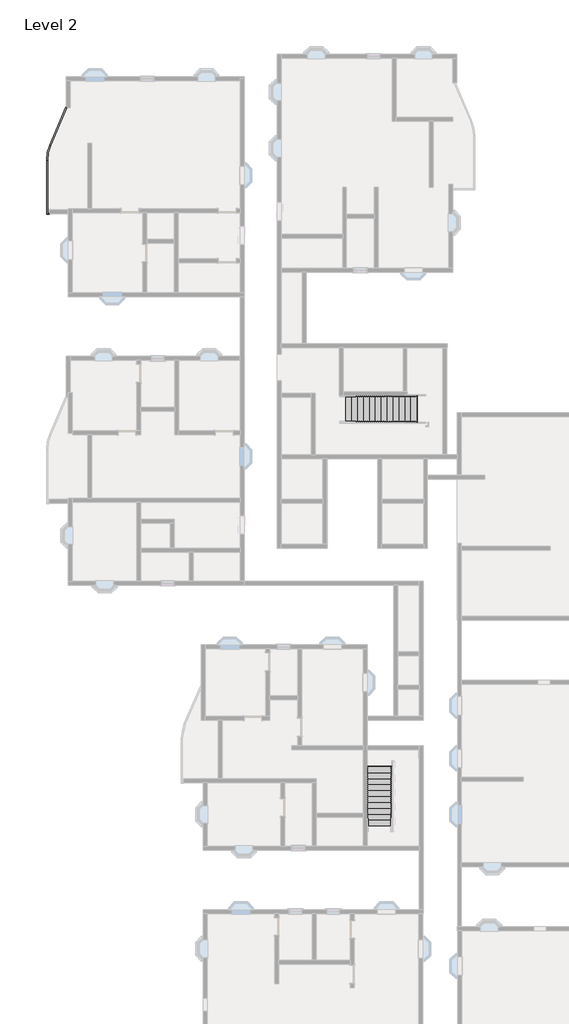
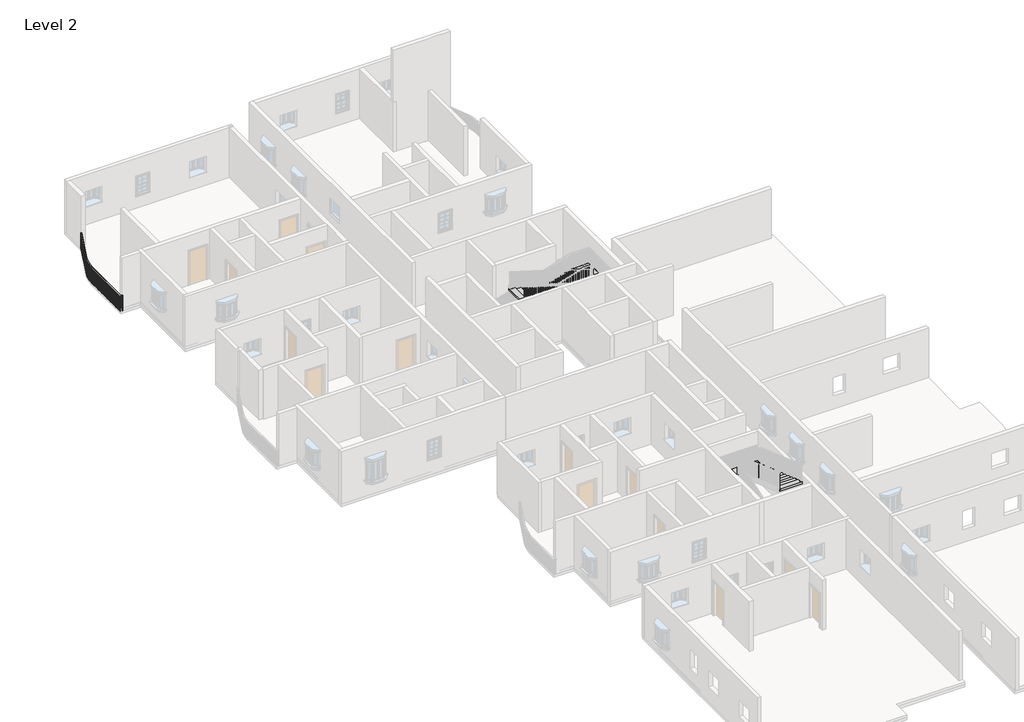
# One storey, part 12 of 14: 2 stair flights, 1 railing.
"""IFC4 building model written with IfcOpenShell, lengths in millimetres."""

from ifc_helpers import new_model, si_unit, frame, origin, place, context, project, spatial, polyline, circle_curve, outline, extrude, transform, mapped, element, save
from ifc_brep_helpers import plane_surface, cylinder_surface, revolved_surface, advanced_brep
from components import stair_flight_f6874503, stair_flight_175a6785

model = new_model("IFC4")

# Units and contexts
model_context = context("Model", 3, world=origin())
ifc_project = project(units=[si_unit("LENGTHUNIT", "METRE", prefix="MILLI")], contexts=[model_context])

# Site, building, storey
site = spatial("IfcSite", under=ifc_project)
building = spatial("IfcBuilding", under=site)
storey = spatial("IfcBuildingStorey", under=building, Name="Level 2", Elevation=3048.0)

# Railing
placement = place(None, origin())
element("IfcRailing", 1, ObjectType="Handrail - Rectangular", at=placement, inside=storey, context=model_context, shape_type="SolidModel", body=[
    advanced_brep(
    [(-19327.739878, 27355.8257339, 3962.4), (-19327.739878, 27355.8257339, 3911.6), (-19374.4383922, 27375.822953, 3911.6), (-19374.4383922, 27375.822953, 3962.4), (-20162.483418, 25406.4905323, 3962.4), (-20162.483418, 25406.4905323, 3911.6), (-20209.1819322, 25426.4877514, 3911.6), (-20209.1819322, 25426.4877514, 3962.4), (-20316.2891351, 24656.5948172, 3911.6), (-20316.2891351, 24656.5948172, 3962.4), (-20367.0891351, 24656.5948172, 3911.6), (-20367.0891351, 24656.5948172, 3962.4), (-20316.2891351, 21915.0583494, 3962.4), (-20316.2891351, 21915.0583494, 3911.6), (-20367.0891351, 21864.2583494, 3911.6), (-20367.0891351, 21864.2583494, 3962.4), (-20240.0891351, 21915.0583494, 3962.4), (-20240.0891351, 21864.2583494, 3962.4), (-20240.0891351, 21864.2583494, 3911.6), (-20240.0891351, 21915.0583494, 3911.6)],
    [
        (0, 1),
        (1, 2),
        (2, 3),
        (3, 0),
        (0, 4),
        (4, 5),
        (5, 1),
        (5, 6),
        (6, 2),
        (6, 7),
        (7, 3),
        (7, 4),
        (8, 5, circle_curve(frame((-18411.2891351, 24656.5948172, 3911.6), z_axis=(0.0, 0.0, -1.0), x_axis=(-0.9192620907623796, 0.39364604467361086, 0.0)), 1905.0)),
        (4, 9, circle_curve(frame((-18411.2891351, 24656.5948172, 3962.4), z_axis=(0.0, 0.0, 1.0), x_axis=(-0.9192620907623796, 0.39364604467361086, 0.0)), 1905.0)),
        (9, 8),
        (10, 6, circle_curve(frame((-18411.2891351, 24656.5948172, 3911.6), z_axis=(0.0, 0.0, -1.0), x_axis=(-0.9192620907623796, 0.39364604467361086, 0.0)), 1955.8)),
        (8, 10),
        (11, 7, circle_curve(frame((-18411.2891351, 24656.5948172, 3962.4), z_axis=(0.0, 0.0, -1.0), x_axis=(-0.9192620907623796, 0.39364604467361086, 0.0)), 1955.8)),
        (10, 11),
        (11, 9),
        (9, 12),
        (12, 13),
        (13, 8),
        (13, 14),
        (14, 10),
        (14, 15),
        (15, 11),
        (15, 12),
        (16, 17),
        (17, 18),
        (18, 19),
        (19, 16),
        (12, 16),
        (19, 13),
        (18, 14),
        (17, 15),
    ],
    [
        plane_surface(frame((-19351.0891351, 27365.8243434, 3962.4), z_axis=(0.3936460446736102, 0.91926209076238, 0.0), x_axis=(0.91926209076238, -0.3936460446736102, 0.0))),
        plane_surface(frame((-19327.739878, 27355.8257339, 3962.4), z_axis=(0.9192620907623803, -0.39364604467360953, 0.0), x_axis=(-0.39364604467360953, -0.9192620907623803, 0.0))),
        plane_surface(frame((-19327.739878, 27355.8257339, 3911.6), z_axis=(0.0, 0.0, -1.0), x_axis=(-0.39364604467360953, -0.9192620907623803, 0.0))),
        plane_surface(frame((-19374.4383922, 27375.822953, 3911.6), z_axis=(-0.9192620907623803, 0.39364604467360953, 0.0), x_axis=(-0.39364604467360953, -0.9192620907623803, 0.0))),
        plane_surface(frame((-19374.4383922, 27375.822953, 3962.4), z_axis=(0.0, 0.0, 1.0), x_axis=(-0.39364604467360953, -0.9192620907623803, 0.0))),
        revolved_surface(polyline([(-20162.48341800233, 25406.49053230323, 3962.4), (-20162.48341800233, 25406.49053230323, 3911.6)]), (-18411.2891351, 24656.5948172, 3962.4), (0.0, 0.0, 1.0)),
        plane_surface(frame((-18411.2891351, 24656.5948172, 3911.6), z_axis=(0.0, 0.0, -1.0000000000000002), x_axis=(-0.9192620907623797, 0.3936460446736109, 0.0))),
        cylinder_surface(frame((-18411.2891351, 24656.5948172, 3962.4), z_axis=(0.0, 0.0, 1.0), x_axis=(-0.9192620907623796, 0.39364604467361086, 0.0)), 1955.8),
        plane_surface(frame((-18411.2891351, 24656.5948172, 3962.4), z_axis=(0.0, 0.0, 1.0000000000000002), x_axis=(-0.9192620907623797, 0.3936460446736109, 0.0))),
        plane_surface(frame((-20316.2891351, 24656.5948172, 3962.4), z_axis=(1.0, 0.0, 0.0), x_axis=(0.0, -1.0, 0.0))),
        plane_surface(frame((-20316.2891351, 24656.5948172, 3911.6), z_axis=(0.0, 0.0, -1.0), x_axis=(0.0, -1.0, 0.0))),
        plane_surface(frame((-20367.0891351, 24656.5948172, 3911.6), z_axis=(-1.0, 0.0, 0.0), x_axis=(0.0, -1.0, 0.0))),
        plane_surface(frame((-20367.0891351, 24656.5948172, 3962.4), z_axis=(0.0, 0.0, 1.0), x_axis=(0.0, -1.0, 0.0))),
        plane_surface(frame((-20240.0891351, 21889.6583494, 3962.4), z_axis=(1.0, 0.0, 0.0), x_axis=(0.0, 1.0, 0.0))),
        plane_surface(frame((-20316.2891351, 21915.0583494, 3962.4), z_axis=(0.0, 1.0, 0.0), x_axis=(1.0, 0.0, 0.0))),
        plane_surface(frame((-20316.2891351, 21915.0583494, 3911.6), z_axis=(0.0, 0.0, -1.0), x_axis=(1.0, 0.0, 0.0))),
        plane_surface(frame((-20367.0891351, 21864.2583494, 3911.6), z_axis=(0.0, -1.0, 0.0), x_axis=(1.0, 0.0, 0.0))),
        plane_surface(frame((-20367.0891351, 21864.2583494, 3962.4), z_axis=(0.0, 0.0, 1.0), x_axis=(1.0, 0.0, 0.0))),
    ],
    [
        (0, [[1, 2, 3, 4]]),
        (1, [[-1, 5, 6, 7]]),
        (2, [[-2, -7, 8, 9]]),
        (3, [[-3, -9, 10, 11]]),
        (4, [[-4, -11, 12, -5]]),
        (5, [[13, -6, 14, 15]]),
        (6, [[16, -8, -13, 17]]),
        (7, [[18, -10, -16, 19]]),
        (8, [[-14, -12, -18, 20]]),
        (9, [[-15, 21, 22, 23]]),
        (10, [[-17, -23, 24, 25]]),
        (11, [[-19, -25, 26, 27]]),
        (12, [[-20, -27, 28, -21]]),
        (13, [[29, 30, 31, 32]]),
        (14, [[-22, 33, -32, 34]]),
        (15, [[-24, -34, -31, 35]]),
        (16, [[-26, -35, -30, 36]]),
        (17, [[-28, -36, -29, -33]]),
    ],
),
    extrude(outline(polyline([(-20351.2141351, 21922.9198172), (-20332.1641351, 21922.9198172), (-20332.1641351, 21903.8698172), (-20351.2141351, 21903.8698172), (-20351.2141351, 21922.9198172)])), frame((0.0, 0.0, 3048.0), z_axis=(0.0, 0.0, 1.0), x_axis=(1.0, 0.0, 0.0)), (0.0, 0.0, 1.0), 863.6),
    extrude(outline(polyline([(-20351.2141351, 22024.5198172), (-20332.1641351, 22024.5198172), (-20332.1641351, 22005.4698172), (-20351.2141351, 22005.4698172), (-20351.2141351, 22024.5198172)])), frame((0.0, 0.0, 3048.0), z_axis=(0.0, 0.0, 1.0), x_axis=(1.0, 0.0, 0.0)), (0.0, 0.0, 1.0), 863.6),
    extrude(outline(polyline([(-20351.2141351, 22126.1198172), (-20332.1641351, 22126.1198172), (-20332.1641351, 22107.0698172), (-20351.2141351, 22107.0698172), (-20351.2141351, 22126.1198172)])), frame((0.0, 0.0, 3048.0), z_axis=(0.0, 0.0, 1.0), x_axis=(1.0, 0.0, 0.0)), (0.0, 0.0, 1.0), 863.6),
    extrude(outline(polyline([(-20351.2141351, 22227.7198172), (-20332.1641351, 22227.7198172), (-20332.1641351, 22208.6698172), (-20351.2141351, 22208.6698172), (-20351.2141351, 22227.7198172)])), frame((0.0, 0.0, 3048.0), z_axis=(0.0, 0.0, 1.0), x_axis=(1.0, 0.0, 0.0)), (0.0, 0.0, 1.0), 863.6),
    extrude(outline(polyline([(-20351.2141351, 22329.3198172), (-20332.1641351, 22329.3198172), (-20332.1641351, 22310.2698172), (-20351.2141351, 22310.2698172), (-20351.2141351, 22329.3198172)])), frame((0.0, 0.0, 3048.0), z_axis=(0.0, 0.0, 1.0), x_axis=(1.0, 0.0, 0.0)), (0.0, 0.0, 1.0), 863.6),
    extrude(outline(polyline([(-20351.2141351, 22430.9198172), (-20332.1641351, 22430.9198172), (-20332.1641351, 22411.8698172), (-20351.2141351, 22411.8698172), (-20351.2141351, 22430.9198172)])), frame((0.0, 0.0, 3048.0), z_axis=(0.0, 0.0, 1.0), x_axis=(1.0, 0.0, 0.0)), (0.0, 0.0, 1.0), 863.6),
    extrude(outline(polyline([(-20351.2141351, 22532.5198172), (-20332.1641351, 22532.5198172), (-20332.1641351, 22513.4698172), (-20351.2141351, 22513.4698172), (-20351.2141351, 22532.5198172)])), frame((0.0, 0.0, 3048.0), z_axis=(0.0, 0.0, 1.0), x_axis=(1.0, 0.0, 0.0)), (0.0, 0.0, 1.0), 863.6),
    extrude(outline(polyline([(-20351.2141351, 22634.1198172), (-20332.1641351, 22634.1198172), (-20332.1641351, 22615.0698172), (-20351.2141351, 22615.0698172), (-20351.2141351, 22634.1198172)])), frame((0.0, 0.0, 3048.0), z_axis=(0.0, 0.0, 1.0), x_axis=(1.0, 0.0, 0.0)), (0.0, 0.0, 1.0), 863.6),
    extrude(outline(polyline([(-20351.2141351, 22735.7198172), (-20332.1641351, 22735.7198172), (-20332.1641351, 22716.6698172), (-20351.2141351, 22716.6698172), (-20351.2141351, 22735.7198172)])), frame((0.0, 0.0, 3048.0), z_axis=(0.0, 0.0, 1.0), x_axis=(1.0, 0.0, 0.0)), (0.0, 0.0, 1.0), 863.6),
    extrude(outline(polyline([(-20351.2141351, 22837.3198172), (-20332.1641351, 22837.3198172), (-20332.1641351, 22818.2698172), (-20351.2141351, 22818.2698172), (-20351.2141351, 22837.3198172)])), frame((0.0, 0.0, 3048.0), z_axis=(0.0, 0.0, 1.0), x_axis=(1.0, 0.0, 0.0)), (0.0, 0.0, 1.0), 863.6),
    extrude(outline(polyline([(-20351.2141351, 22938.9198172), (-20332.1641351, 22938.9198172), (-20332.1641351, 22919.8698172), (-20351.2141351, 22919.8698172), (-20351.2141351, 22938.9198172)])), frame((0.0, 0.0, 3048.0), z_axis=(0.0, 0.0, 1.0), x_axis=(1.0, 0.0, 0.0)), (0.0, 0.0, 1.0), 863.6),
    extrude(outline(polyline([(-20351.2141351, 23040.5198172), (-20332.1641351, 23040.5198172), (-20332.1641351, 23021.4698172), (-20351.2141351, 23021.4698172), (-20351.2141351, 23040.5198172)])), frame((0.0, 0.0, 3048.0), z_axis=(0.0, 0.0, 1.0), x_axis=(1.0, 0.0, 0.0)), (0.0, 0.0, 1.0), 863.6),
    extrude(outline(polyline([(-20351.2141351, 23142.1198172), (-20332.1641351, 23142.1198172), (-20332.1641351, 23123.0698172), (-20351.2141351, 23123.0698172), (-20351.2141351, 23142.1198172)])), frame((0.0, 0.0, 3048.0), z_axis=(0.0, 0.0, 1.0), x_axis=(1.0, 0.0, 0.0)), (0.0, 0.0, 1.0), 863.6),
    extrude(outline(polyline([(-20351.2141351, 23243.7198172), (-20332.1641351, 23243.7198172), (-20332.1641351, 23224.6698172), (-20351.2141351, 23224.6698172), (-20351.2141351, 23243.7198172)])), frame((0.0, 0.0, 3048.0), z_axis=(0.0, 0.0, 1.0), x_axis=(1.0, 0.0, 0.0)), (0.0, 0.0, 1.0), 863.6),
    extrude(outline(polyline([(-20351.2141351, 23345.3198172), (-20332.1641351, 23345.3198172), (-20332.1641351, 23326.2698172), (-20351.2141351, 23326.2698172), (-20351.2141351, 23345.3198172)])), frame((0.0, 0.0, 3048.0), z_axis=(0.0, 0.0, 1.0), x_axis=(1.0, 0.0, 0.0)), (0.0, 0.0, 1.0), 863.6),
    extrude(outline(polyline([(-20351.2141351, 23446.9198172), (-20332.1641351, 23446.9198172), (-20332.1641351, 23427.8698172), (-20351.2141351, 23427.8698172), (-20351.2141351, 23446.9198172)])), frame((0.0, 0.0, 3048.0), z_axis=(0.0, 0.0, 1.0), x_axis=(1.0, 0.0, 0.0)), (0.0, 0.0, 1.0), 863.6),
    extrude(outline(polyline([(-20351.2141351, 23548.5198172), (-20332.1641351, 23548.5198172), (-20332.1641351, 23529.4698172), (-20351.2141351, 23529.4698172), (-20351.2141351, 23548.5198172)])), frame((0.0, 0.0, 3048.0), z_axis=(0.0, 0.0, 1.0), x_axis=(1.0, 0.0, 0.0)), (0.0, 0.0, 1.0), 863.6),
    extrude(outline(polyline([(-20351.2141351, 23650.1198172), (-20332.1641351, 23650.1198172), (-20332.1641351, 23631.0698172), (-20351.2141351, 23631.0698172), (-20351.2141351, 23650.1198172)])), frame((0.0, 0.0, 3048.0), z_axis=(0.0, 0.0, 1.0), x_axis=(1.0, 0.0, 0.0)), (0.0, 0.0, 1.0), 863.6),
    extrude(outline(polyline([(-20351.2141351, 23751.7198172), (-20332.1641351, 23751.7198172), (-20332.1641351, 23732.6698172), (-20351.2141351, 23732.6698172), (-20351.2141351, 23751.7198172)])), frame((0.0, 0.0, 3048.0), z_axis=(0.0, 0.0, 1.0), x_axis=(1.0, 0.0, 0.0)), (0.0, 0.0, 1.0), 863.6),
    extrude(outline(polyline([(-20351.2141351, 23853.3198172), (-20332.1641351, 23853.3198172), (-20332.1641351, 23834.2698172), (-20351.2141351, 23834.2698172), (-20351.2141351, 23853.3198172)])), frame((0.0, 0.0, 3048.0), z_axis=(0.0, 0.0, 1.0), x_axis=(1.0, 0.0, 0.0)), (0.0, 0.0, 1.0), 863.6),
    extrude(outline(polyline([(-20351.2141351, 23954.9198172), (-20332.1641351, 23954.9198172), (-20332.1641351, 23935.8698172), (-20351.2141351, 23935.8698172), (-20351.2141351, 23954.9198172)])), frame((0.0, 0.0, 3048.0), z_axis=(0.0, 0.0, 1.0), x_axis=(1.0, 0.0, 0.0)), (0.0, 0.0, 1.0), 863.6),
    extrude(outline(polyline([(-20351.2141351, 24056.5198172), (-20332.1641351, 24056.5198172), (-20332.1641351, 24037.4698172), (-20351.2141351, 24037.4698172), (-20351.2141351, 24056.5198172)])), frame((0.0, 0.0, 3048.0), z_axis=(0.0, 0.0, 1.0), x_axis=(1.0, 0.0, 0.0)), (0.0, 0.0, 1.0), 863.6),
    extrude(outline(polyline([(-20351.2141351, 24158.1198172), (-20332.1641351, 24158.1198172), (-20332.1641351, 24139.0698172), (-20351.2141351, 24139.0698172), (-20351.2141351, 24158.1198172)])), frame((0.0, 0.0, 3048.0), z_axis=(0.0, 0.0, 1.0), x_axis=(1.0, 0.0, 0.0)), (0.0, 0.0, 1.0), 863.6),
    extrude(outline(polyline([(-20351.2141351, 24259.7198172), (-20332.1641351, 24259.7198172), (-20332.1641351, 24240.6698172), (-20351.2141351, 24240.6698172), (-20351.2141351, 24259.7198172)])), frame((0.0, 0.0, 3048.0), z_axis=(0.0, 0.0, 1.0), x_axis=(1.0, 0.0, 0.0)), (0.0, 0.0, 1.0), 863.6),
    extrude(outline(polyline([(-20351.2141351, 24361.3198172), (-20332.1641351, 24361.3198172), (-20332.1641351, 24342.2698172), (-20351.2141351, 24342.2698172), (-20351.2141351, 24361.3198172)])), frame((0.0, 0.0, 3048.0), z_axis=(0.0, 0.0, 1.0), x_axis=(1.0, 0.0, 0.0)), (0.0, 0.0, 1.0), 863.6),
    extrude(outline(polyline([(-20351.2141351, 24462.9198172), (-20332.1641351, 24462.9198172), (-20332.1641351, 24443.8698172), (-20351.2141351, 24443.8698172), (-20351.2141351, 24462.9198172)])), frame((0.0, 0.0, 3048.0), z_axis=(0.0, 0.0, 1.0), x_axis=(1.0, 0.0, 0.0)), (0.0, 0.0, 1.0), 863.6),
    extrude(outline(polyline([(-20351.2141351, 24564.5198172), (-20332.1641351, 24564.5198172), (-20332.1641351, 24545.4698172), (-20351.2141351, 24545.4698172), (-20351.2141351, 24564.5198172)])), frame((0.0, 0.0, 3048.0), z_axis=(0.0, 0.0, 1.0), x_axis=(1.0, 0.0, 0.0)), (0.0, 0.0, 1.0), 863.6),
    extrude(outline(polyline([(-20349.6005818, 24736.2720848), (-20330.5630441, 24735.5831307), (-20331.2519982, 24716.545593), (-20350.289536, 24717.2345471), (-20349.6005818, 24736.2720848)])), frame((0.0, 0.0, 3048.0), z_axis=(0.0, 0.0, 1.0), x_axis=(1.0, 0.0, 0.0)), (0.0, 0.0, 1.0), 863.6),
    extrude(outline(polyline([(-20342.724955, 24838.1310534), (-20323.750023, 24836.4415402), (-20325.4395363, 24817.4666081), (-20344.4144683, 24819.1561214), (-20342.724955, 24838.1310534)])), frame((0.0, 0.0, 3048.0), z_axis=(0.0, 0.0, 1.0), x_axis=(1.0, 0.0, 0.0)), (0.0, 0.0, 1.0), 863.6),
    extrude(outline(polyline([(-20330.5003254, 24939.4872677), (-20311.6405491, 24936.8018743), (-20314.3259425, 24917.942098), (-20333.1857188, 24920.6274914), (-20330.5003254, 24939.4872677)])), frame((0.0, 0.0, 3048.0), z_axis=(0.0, 0.0, 1.0), x_axis=(1.0, 0.0, 0.0)), (0.0, 0.0, 1.0), 863.6),
    extrude(outline(polyline([(-20312.9605484, 25040.0600272), (-20294.2681589, 25036.3861907), (-20297.9419954, 25017.6938012), (-20316.6343849, 25021.3676377), (-20312.9605484, 25040.0600272)])), frame((0.0, 0.0, 3048.0), z_axis=(0.0, 0.0, 1.0), x_axis=(1.0, 0.0, 0.0)), (0.0, 0.0, 1.0), 863.6),
    extrude(outline(polyline([(-20290.1541995, 25139.5708014), (-20271.6809643, 25134.9186963), (-20276.3330693, 25116.4454611), (-20294.8063045, 25121.0975662), (-20290.1541995, 25139.5708014)])), frame((0.0, 0.0, 3048.0), z_axis=(0.0, 0.0, 1.0), x_axis=(1.0, 0.0, 0.0)), (0.0, 0.0, 1.0), 863.6),
    extrude(outline(polyline([(-20262.1444395, 25237.7440008), (-20243.9415192, 25232.1265109), (-20249.5590091, 25213.9235906), (-20267.7619294, 25219.5410805), (-20262.1444395, 25237.7440008)])), frame((0.0, 0.0, 3048.0), z_axis=(0.0, 0.0, 1.0), x_axis=(1.0, 0.0, 0.0)), (0.0, 0.0, 1.0), 863.6),
    extrude(outline(polyline([(-20229.0088399, 25334.3077402), (-20211.1266465, 25327.7404228), (-20217.693964, 25309.8582293), (-20235.5761574, 25316.4255468), (-20229.0088399, 25334.3077402)])), frame((0.0, 0.0, 3048.0), z_axis=(0.0, 0.0, 1.0), x_axis=(1.0, 0.0, 0.0)), (0.0, 0.0, 1.0), 863.6),
    extrude(outline(polyline([(-20155.9843907, 25510.389225), (-20138.4724479, 25502.8902678), (-20145.9714051, 25485.378325), (-20163.4833479, 25492.8772822), (-20155.9843907, 25510.389225)])), frame((0.0, 0.0, 3048.0), z_axis=(0.0, 0.0, 1.0), x_axis=(1.0, 0.0, 0.0)), (0.0, 0.0, 1.0), 863.6),
    extrude(outline(polyline([(-20115.9899526, 25603.7862534), (-20098.4780098, 25596.2872963), (-20105.9769669, 25578.7753534), (-20123.4889098, 25586.2743106), (-20115.9899526, 25603.7862534)])), frame((0.0, 0.0, 3048.0), z_axis=(0.0, 0.0, 1.0), x_axis=(1.0, 0.0, 0.0)), (0.0, 0.0, 1.0), 863.6),
    extrude(outline(polyline([(-20075.9955145, 25697.1832818), (-20058.4835716, 25689.6843247), (-20065.9825288, 25672.1723818), (-20083.4944716, 25679.671339), (-20075.9955145, 25697.1832818)])), frame((0.0, 0.0, 3048.0), z_axis=(0.0, 0.0, 1.0), x_axis=(1.0, 0.0, 0.0)), (0.0, 0.0, 1.0), 863.6),
    extrude(outline(polyline([(-20036.0010763, 25790.5803103), (-20018.4891335, 25783.0813531), (-20025.9880906, 25765.5694103), (-20043.5000335, 25773.0683674), (-20036.0010763, 25790.5803103)])), frame((0.0, 0.0, 3048.0), z_axis=(0.0, 0.0, 1.0), x_axis=(1.0, 0.0, 0.0)), (0.0, 0.0, 1.0), 863.6),
    extrude(outline(polyline([(-19996.0066382, 25883.9773387), (-19978.4946954, 25876.4783815), (-19985.9936525, 25858.9664387), (-20003.5055953, 25866.4653958), (-19996.0066382, 25883.9773387)])), frame((0.0, 0.0, 3048.0), z_axis=(0.0, 0.0, 1.0), x_axis=(1.0, 0.0, 0.0)), (0.0, 0.0, 1.0), 863.6),
    extrude(outline(polyline([(-19956.0122, 25977.3743671), (-19938.5002572, 25969.8754099), (-19945.9992144, 25952.3634671), (-19963.5111572, 25959.8624243), (-19956.0122, 25977.3743671)])), frame((0.0, 0.0, 3048.0), z_axis=(0.0, 0.0, 1.0), x_axis=(1.0, 0.0, 0.0)), (0.0, 0.0, 1.0), 863.6),
    extrude(outline(polyline([(-19916.0177619, 26070.7713955), (-19898.5058191, 26063.2724384), (-19906.0047762, 26045.7604955), (-19923.5167191, 26053.2594527), (-19916.0177619, 26070.7713955)])), frame((0.0, 0.0, 3048.0), z_axis=(0.0, 0.0, 1.0), x_axis=(1.0, 0.0, 0.0)), (0.0, 0.0, 1.0), 863.6),
    extrude(outline(polyline([(-19876.0233238, 26164.1684239), (-19858.5113809, 26156.6694668), (-19866.0103381, 26139.157524), (-19883.5222809, 26146.6564811), (-19876.0233238, 26164.1684239)])), frame((0.0, 0.0, 3048.0), z_axis=(0.0, 0.0, 1.0), x_axis=(1.0, 0.0, 0.0)), (0.0, 0.0, 1.0), 863.6),
    extrude(outline(polyline([(-19836.0288856, 26257.5654524), (-19818.5169428, 26250.0664952), (-19826.0159, 26232.5545524), (-19843.5278428, 26240.0535095), (-19836.0288856, 26257.5654524)])), frame((0.0, 0.0, 3048.0), z_axis=(0.0, 0.0, 1.0), x_axis=(1.0, 0.0, 0.0)), (0.0, 0.0, 1.0), 863.6),
    extrude(outline(polyline([(-19796.0344475, 26350.9624808), (-19778.5225047, 26343.4635236), (-19786.0214618, 26325.9515808), (-19803.5334046, 26333.450538), (-19796.0344475, 26350.9624808)])), frame((0.0, 0.0, 3048.0), z_axis=(0.0, 0.0, 1.0), x_axis=(1.0, 0.0, 0.0)), (0.0, 0.0, 1.0), 863.6),
    extrude(outline(polyline([(-19756.0400094, 26444.3595092), (-19738.5280665, 26436.860552), (-19746.0270237, 26419.3486092), (-19763.5389665, 26426.8475664), (-19756.0400094, 26444.3595092)])), frame((0.0, 0.0, 3048.0), z_axis=(0.0, 0.0, 1.0), x_axis=(1.0, 0.0, 0.0)), (0.0, 0.0, 1.0), 863.6),
    extrude(outline(polyline([(-19716.0455712, 26537.7565376), (-19698.5336284, 26530.2575805), (-19706.0325855, 26512.7456376), (-19723.5445284, 26520.2445948), (-19716.0455712, 26537.7565376)])), frame((0.0, 0.0, 3048.0), z_axis=(0.0, 0.0, 1.0), x_axis=(1.0, 0.0, 0.0)), (0.0, 0.0, 1.0), 863.6),
    extrude(outline(polyline([(-19676.0511331, 26631.153566), (-19658.5391902, 26623.6546089), (-19666.0381474, 26606.1426661), (-19683.5500902, 26613.6416232), (-19676.0511331, 26631.153566)])), frame((0.0, 0.0, 3048.0), z_axis=(0.0, 0.0, 1.0), x_axis=(1.0, 0.0, 0.0)), (0.0, 0.0, 1.0), 863.6),
    extrude(outline(polyline([(-19636.0566949, 26724.5505945), (-19618.5447521, 26717.0516373), (-19626.0437093, 26699.5396945), (-19643.5556521, 26707.0386516), (-19636.0566949, 26724.5505945)])), frame((0.0, 0.0, 3048.0), z_axis=(0.0, 0.0, 1.0), x_axis=(1.0, 0.0, 0.0)), (0.0, 0.0, 1.0), 863.6),
    extrude(outline(polyline([(-19596.0622568, 26817.9476229), (-19578.550314, 26810.4486657), (-19586.0492711, 26792.9367229), (-19603.561214, 26800.4356801), (-19596.0622568, 26817.9476229)])), frame((0.0, 0.0, 3048.0), z_axis=(0.0, 0.0, 1.0), x_axis=(1.0, 0.0, 0.0)), (0.0, 0.0, 1.0), 863.6),
    extrude(outline(polyline([(-19556.0678187, 26911.3446513), (-19538.5558758, 26903.8456942), (-19546.054833, 26886.3337513), (-19563.5667758, 26893.8327085), (-19556.0678187, 26911.3446513)])), frame((0.0, 0.0, 3048.0), z_axis=(0.0, 0.0, 1.0), x_axis=(1.0, 0.0, 0.0)), (0.0, 0.0, 1.0), 863.6),
    extrude(outline(polyline([(-19516.0733805, 27004.7416797), (-19498.5614377, 26997.2427226), (-19506.0603948, 26979.7307797), (-19523.5723377, 26987.2297369), (-19516.0733805, 27004.7416797)])), frame((0.0, 0.0, 3048.0), z_axis=(0.0, 0.0, 1.0), x_axis=(1.0, 0.0, 0.0)), (0.0, 0.0, 1.0), 863.6),
    extrude(outline(polyline([(-19476.0789424, 27098.1387082), (-19458.5669996, 27090.639751), (-19466.0659567, 27073.1278082), (-19483.5778995, 27080.6267653), (-19476.0789424, 27098.1387082)])), frame((0.0, 0.0, 3048.0), z_axis=(0.0, 0.0, 1.0), x_axis=(1.0, 0.0, 0.0)), (0.0, 0.0, 1.0), 863.6),
    extrude(outline(polyline([(-19436.0845042, 27191.5357366), (-19418.5725614, 27184.0367794), (-19426.0715186, 27166.5248366), (-19443.5834614, 27174.0237937), (-19436.0845042, 27191.5357366)])), frame((0.0, 0.0, 3048.0), z_axis=(0.0, 0.0, 1.0), x_axis=(1.0, 0.0, 0.0)), (0.0, 0.0, 1.0), 863.6),
    extrude(outline(polyline([(-19396.0900661, 27284.932765), (-19378.5781233, 27277.4338078), (-19386.0770804, 27259.921865), (-19403.5890233, 27267.4208222), (-19396.0900661, 27284.932765)])), frame((0.0, 0.0, 3048.0), z_axis=(0.0, 0.0, 1.0), x_axis=(1.0, 0.0, 0.0)), (0.0, 0.0, 1.0), 863.6),
    extrude(outline(polyline([(-20351.2141351, 21899.1833494), (-20332.1641351, 21899.1833494), (-20332.1641351, 21880.1333494), (-20351.2141351, 21880.1333494), (-20351.2141351, 21899.1833494)])), frame((0.0, 0.0, 3048.0), z_axis=(0.0, 0.0, 1.0), x_axis=(1.0, 0.0, 0.0)), (0.0, 0.0, 1.0), 863.6),
    extrude(outline(polyline([(-20351.2141351, 24666.1198172), (-20332.1641351, 24666.1198172), (-20332.1641351, 24647.0698172), (-20351.2141351, 24647.0698172), (-20351.2141351, 24666.1198172)])), frame((0.0, 0.0, 3048.0), z_axis=(0.0, 0.0, 1.0), x_axis=(1.0, 0.0, 0.0)), (0.0, 0.0, 1.0), 863.6),
    extrude(outline(polyline([(-20190.839168, 25428.9945919), (-20173.3272251, 25421.4956347), (-20180.8261823, 25403.9836919), (-20198.3381251, 25411.482649), (-20190.839168, 25428.9945919)])), frame((0.0, 0.0, 3048.0), z_axis=(0.0, 0.0, 1.0), x_axis=(1.0, 0.0, 0.0)), (0.0, 0.0, 1.0), 863.6),
    extrude(outline(polyline([(-20259.1391351, 21880.1333494), (-20259.1391351, 21899.1833494), (-20240.0891351, 21899.1833494), (-20240.0891351, 21880.1333494), (-20259.1391351, 21880.1333494)])), frame((0.0, 0.0, 3048.0), z_axis=(0.0, 0.0, 1.0), x_axis=(1.0, 0.0, 0.0)), (0.0, 0.0, 1.0), 863.6),
    extrude(outline(polyline([(-19359.8451065, 27369.573822), (-19342.3331637, 27362.0748648), (-19349.8321209, 27344.562922), (-19367.3440637, 27352.0618792), (-19359.8451065, 27369.573822)])), frame((0.0, 0.0, 3048.0), z_axis=(0.0, 0.0, 1.0), x_axis=(1.0, 0.0, 0.0)), (0.0, 0.0, 1.0), 863.6),
])

# Stair flights
stair_flight_shape = stair_flight_f6874503(model_context)
element("IfcStairFlight", 2, ObjectType="2\" Tread 1\" Nosing 1/4\" Riser", at=placement, inside=storey, context=model_context, shape_type="MappedRepresentation", body=[
    mapped(stair_flight_shape, transform((0.0, 0.0, 0.0), x_axis=(1.0, 0.0, 0.0), y_axis=(0.0, 1.0, 0.0), z_axis=(0.0, 0.0, 1.0))),
])
stair_flight_2_shape = stair_flight_175a6785(model_context)
element("IfcStairFlight", 3, ObjectType="2\" Tread 1\" Nosing 1/4\" Riser", at=placement, inside=storey, context=model_context, shape_type="MappedRepresentation", body=[
    mapped(stair_flight_2_shape, transform((0.0, 0.0, 0.0), x_axis=(1.0, 0.0, 0.0), y_axis=(0.0, 1.0, 0.0), z_axis=(0.0, 0.0, 1.0))),
])

save(model, "model.ifc")

# Revit data of these elements
# Type "Handrail - Rectangular"
#   Assembly Code = "C2010400"
#   built-in parameter 1008612 = 0.0416667 (stored number, unit not read)
#   built-in parameter 1008611 = 0.0416667 (stored number, unit not read)
#   built-in parameter 1008609 = 0.333333 (stored number, unit not read)
#   built-in parameter 1008604 = 0.166667 (stored number, unit not read)
#   built-in parameter 1008603 = 0.166667 (stored number, unit not read)
#   Railing Height = 3' - 0"
#   built-in parameter 1008630 = 2
#   built-in parameter 1008610 = 2
#   built-in parameter 1008618 = Baluster - Square : 3/4"
# Element 1 (IfcRailing, "Handrail - Rectangular")
#   Phase Created = New Construction
# Elements 2, 3 (IfcStairFlight, "2\" Tread 1\" Nosing 1/4\" Riser")
#   Phase Created = New Construction
